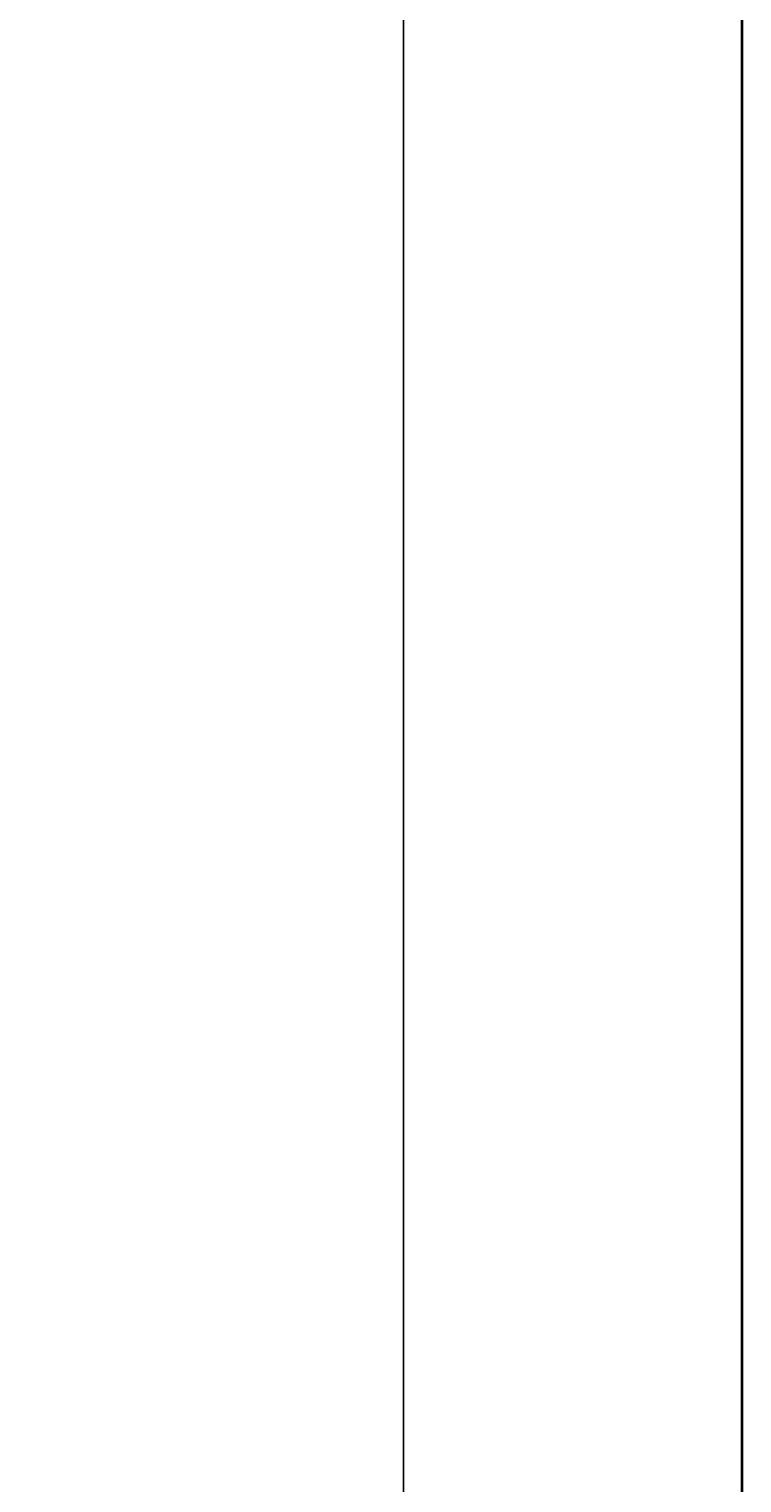
# Model space of a CAD drawing. Units: inches. Extents: x 1885 to 2748, y 783 to 2421.
# Tile 116 of 117: x 2618 to 2748, y 1850 to 2115. Entities that reach past the tile are written whole.
import ezdxf

# ---------------------------------------------------------------- set-up
doc = ezdxf.new("R2010")
doc.units = ezdxf.units.IN
doc.layers.add('A-ANNO-DIMS', color=2, linetype='Continuous', lineweight=18)
doc.layers.add('A-ANNO-TTLB', color=7, linetype='Continuous', lineweight=35)
doc.styles.get("Standard").update_dxf_attribs({"font": 'arial.ttf'})
doc.dimstyles.get("Standard").update_dxf_attribs({"dimtxt": 0.18, "dimasz": 0.18, "dimexe": 0.18, "dimexo": 0.0625, "dimgap": 0.09, "dimtad": 0, "dimtih": 1, "dimtoh": 1, "dimdec": 4, "dimzin": 0, "dimdsep": 46, "dimtxsty": 'Standard', "dimcen": 0.09, "dimadec": 0, "dimazin": 0, "dimtfac": 1, "dimtdec": 4, "dimtofl": 0, "dimtmove": 0, "dimatfit": 3, "dimfxl": 1, "dimtolj": 1, "dimtzin": 0, "dimarcsym": 0})

# ---------------------------------------------------------------- blocks, each defined once
blk = doc.blocks.new('*D44')
at = {"layer": 'A-ANNO-DIMS', "color": 0, "lineweight": -2, "transparency": 16777216}
for p, q in [((2618.34, 2352.51), (2686.7, 2352.51)), ((2686.52, 2352.33), (2686.52, 1705.19)), ((2686.52, 1057.69), (2686.52, 1704.82)), ((2618.34, 1057.51), (2686.7, 1057.51))]:
    blk.add_line(p, q, dxfattribs=at)
at = {"layer": 'A-ANNO-DIMS', "color": 0, "transparency": 16777216}
for points in [[(2686.49, 2352.33), (2686.55, 2352.33), (2686.52, 2352.51)], [(2686.49, 1057.69), (2686.55, 1057.69), (2686.52, 1057.51)]]:
    blk.add_solid(points, dxfattribs=at)
at = {"layer": 'Defpoints', "color": 0, "transparency": 16777216}
for p in [(2618.27, 2352.51), (2686.52, 2352.51), (2618.27, 1057.51)]:
    blk.add_point(p, dxfattribs=at)
at = {"layer": 'A-ANNO-DIMS', "color": 0, "transparency": 16777216, "insert": (2686.52, 1705.01), "char_height": 0.18, "attachment_point": 5}
blk.add_mtext('\\A1;1295', dxfattribs=at)

msp = doc.modelspace()

# ---------------------------------------------------------------- linework, layer by layer
at = {"layer": 'A-ANNO-TTLB'}
msp.add_lwpolyline([(1885.16, 2409.17), (2748.2, 2409.17), (2748.2, 922.58), (1885.16, 922.58)], close=True, dxfattribs=at)

# ---------------------------------------------------------------- dimensions: what is measured, and where the dimension line sits
at = {"layer": 'A-ANNO-DIMS'}
dim = msp.add_linear_dim(base=(2686.52, 2352.51), p1=(2618.27, 1057.51), p2=(2618.27, 2352.51), angle=90, dimstyle='Standard', override={"dimdec": 0, "dimlfac": 1, "dimrnd": 0, "dimzin": 0, "dimdsep": 46, "dimlunit": 2}, dxfattribs=at)
dim.commit()
dim.dimension.update_dxf_attribs({"geometry": '*D44', "text_midpoint": (2686.52, 1705.01)})

doc.saveas('drawing.dxf')
